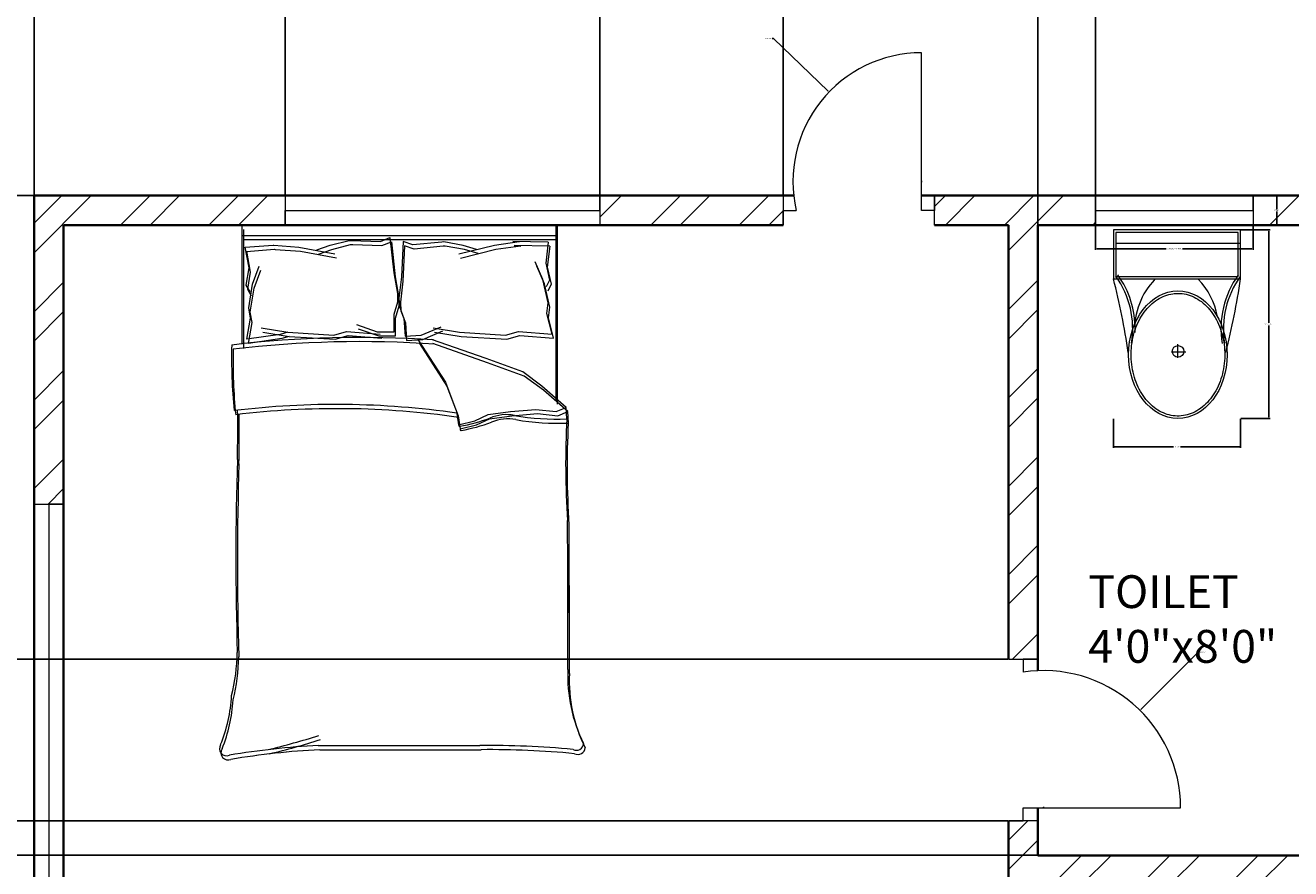
# Model space of a CAD drawing. Units: inches. Extents: x 392 to 1254, y 1207 to 2665.
# Tile 9 of 15: x 540 to 733, y 2127 to 2255. Entities that reach past the tile are written whole.
import ezdxf

# ---------------------------------------------------------------- set-up
doc = ezdxf.new("R2010")
doc.units = ezdxf.units.IN
for name, color, linetype, lineweight in [('A-ANNO-DIMS', 2, 'Continuous', 18), ('A-AREA-IDEN', 7, 'Continuous', 18), ('A-DOOR', 3, 'Continuous', 18), ('A-FLOR-FIXT', 9, 'Continuous', 18), ('A-FURN', 8, 'Continuous', 13), ('A-GLAZ', 4, 'Continuous', 18), ('A-WALL', 7, 'Continuous', 35), ('A-WALL-PATT', 252, 'Continuous', 13)]:
    doc.layers.add(name, color=color, linetype=linetype, lineweight=lineweight)
doc.styles.get("Standard").update_dxf_attribs({"font": 'arial.ttf'})
doc.dimstyles.get("Standard").update_dxf_attribs({"dimtxt": 0.18, "dimasz": 0.18, "dimexe": 0.18, "dimexo": 0.0625, "dimgap": 0.09, "dimtad": 0, "dimtih": 1, "dimtoh": 1, "dimdec": 4, "dimzin": 0, "dimdsep": 46, "dimtxsty": 'Standard', "dimcen": 0.09, "dimadec": 0, "dimazin": 0, "dimtfac": 1, "dimtdec": 4, "dimtofl": 0, "dimtmove": 0, "dimatfit": 3, "dimfxl": 1, "dimtolj": 1, "dimtzin": 0, "dimarcsym": 0})

# ---------------------------------------------------------------- blocks, each defined once
blk = doc.blocks.new('A$C31115884')
for p, q in [((257.5, 466.4), (257.5, 523.2)), ((283.1, 497.7), (223.4, 497.7)), ((0, 200), (0, 0)), ((520, 200), (0, 200)), ((10, 190), (10, 10)), ((510, 190), (10, 190)), ((510, 10), (510, 190)), ((520, 0), (520, 200)), ((510, 54.5), (0, 54.5)), ((10, 10), (510, 10)), ((0, 0), (520, 0))]:
    blk.add_line(p, q)
blk.add_circle((255.6, 496.4), 23.6)
for centre, radius, start, end in [((2777.7, -204.6), 2807, 165.4549, 171.7133), ((3237, 905), 2807, 188.2867, 194.5451), ((-294.5, 403.3), 364.7, 324.2091, 9.3499), ((-294.5, 403.3), 374.7, 324.2091, 9.3499), ((139.5, 406.2), 293.5, 315.8436, 2.6563), ((805.8, 403.3), 364.7, 170.6501, 215.7909), ((805.8, 403.3), 374.7, 179.2036, 215.7909), ((383.6, 406.2), 293.5, 190.2774, 224.1564)]:
    blk.add_arc(centre, radius, start, end)
blk.add_ellipse((256.2, 509.9), major_axis=(0, -260.7), ratio=0.772727)
blk.add_open_spline([(256.2, 259.2), (263.1, 259.2), (270, 259.7), (287.8, 262.3), (298.7, 265.1), (319.9, 273.1), (330.2, 278.4), (350.1, 291.1), (359.7, 298.7), (377.7, 315.9), (386.2, 325.5), (401.7, 346.6), (408.8, 358.1), (421.3, 382.5), (426.8, 395.5), (435.9, 422.4), (439.5, 436.4), (444.8, 465.1), (446.5, 479.7), (447.9, 509.2), (447.6, 524), (445, 553.3), (442.7, 567.8), (436.3, 596), (432.1, 609.7), (421.9, 636), (416, 648.6), (402.5, 672.1), (395, 683), (378.6, 703), (369.8, 712.1), (351.1, 728), (341.3, 734.8), (320.9, 746.2), (310.4, 750.7), (288.9, 757.3), (278, 759.4), (256, 761), (245, 760.6), (223.1, 757.2), (212.3, 754.3), (191.1, 746.1), (180.8, 740.7), (160.9, 727.8), (151.4, 720.1), (133.5, 702.7), (125.1, 693), (109.6, 671.7), (102.6, 660.2), (90.2, 635.7), (84.9, 622.7), (76, 595.6), (72.4, 581.6), (67.2, 552.9), (65.6, 538.2), (64.4, 508.8), (64.8, 494), (67.5, 464.7), (69.9, 450.2), (76.6, 422), (80.8, 408.3), (91.1, 382.2), (97.2, 369.7), (110.8, 346.3), (118.4, 335.4), (134.8, 315.6), (143.7, 306.7), (162.4, 290.9), (172.3, 284.2), (192.8, 273), (203.3, 268.6), (224.8, 262.2), (235.8, 260.2), (249.9, 259.3), (253, 259.2), (256.2, 259.2)], degree=3, knots=[0, 0, 0, 0, 0.110105, 0.110105, 0.285049, 0.285049, 0.459994, 0.459994, 0.634938, 0.634938, 0.809882, 0.809882, 0.984827, 0.984827, 1.159771, 1.159771, 1.334715, 1.334715, 1.50966, 1.50966, 1.684604, 1.684604, 1.859549, 1.859549, 2.034493, 2.034493, 2.209437, 2.209437, 2.384382, 2.384382, 2.559326, 2.559326, 2.73427, 2.73427, 2.909215, 2.909215, 3.084159, 3.084159, 3.259103, 3.259103, 3.434048, 3.434048, 3.608992, 3.608992, 3.783936, 3.783936, 3.958881, 3.958881, 4.133825, 4.133825, 4.30877, 4.30877, 4.483714, 4.483714, 4.658658, 4.658658, 4.833603, 4.833603, 5.008547, 5.008547, 5.183491, 5.183491, 5.358436, 5.358436, 5.53338, 5.53338, 5.708324, 5.708324, 5.883269, 5.883269, 6.058213, 6.058213, 6.233158, 6.233158, 6.283185, 6.283185, 6.283185, 6.283185])
blk = doc.blocks.new('BED-DOUBLE')
for p, q in [((3.47, 63.33), (3.47, 81.44)), ((3.48, 63.33), (3.48, 81.44)), ((51.27, 81.44), (51.27, 54.83)), ((51.27, 81.44), (51.27, 54.83)), ((51.49, 81.44), (51.49, 80.8)), ((3.47, 79.91), (51.27, 79.91)), ((3.48, 79.91), (51.27, 79.91)), ((3.7, 62.69), (3.7, 80.8)), ((3.7, 62.69), (3.7, 80.8)), ((3.7, 79.27), (51.49, 79.27)), ((3.7, 79.27), (51.49, 79.27)), ((16.88, 78.42), (19.77, 79.14)), ((16.88, 78.42), (19.77, 79.14)), ((19.77, 79.14), (20.09, 79.14)), ((19.77, 79.14), (20.09, 79.14)), ((20.09, 79.14), (24.54, 78.99)), ((20.09, 79.14), (24.54, 78.99)), ((24.54, 78.99), (25.98, 79.57)), ((24.54, 78.99), (25.98, 79.57)), ((25.98, 79.57), (26.56, 74.22)), ((25.98, 79.57), (26.56, 74.22)), ((51.49, 80.8), (51.49, 54.19)), ((51.49, 80.8), (51.49, 54.19)), ((3.89, 78.13), (4.47, 74.95)), ((3.89, 78.13), (4.47, 74.95)), ((3.9, 78.1), (8.18, 78.43)), ((3.9, 78.1), (8.18, 78.43)), ((4.12, 77.49), (4.7, 74.31)), ((4.12, 77.49), (4.7, 74.31)), ((4.13, 77.47), (8.41, 77.79)), ((4.13, 77.47), (8.41, 77.79)), ((8.18, 78.43), (8.28, 78.42)), ((8.18, 78.43), (8.28, 78.42)), ((8.28, 78.42), (12.11, 78.13)), ((8.28, 78.42), (12.11, 78.13)), ((8.41, 77.79), (8.51, 77.78)), ((8.41, 77.79), (8.51, 77.78)), ((8.51, 77.78), (12.34, 77.49)), ((8.51, 77.78), (12.34, 77.49)), ((12.11, 78.13), (17.6, 77.11)), ((12.11, 78.13), (17.6, 77.11)), ((12.34, 77.49), (17.83, 76.48)), ((12.34, 77.49), (17.83, 76.48)), ((14.85, 77.69), (16.88, 78.42)), ((14.85, 77.69), (16.88, 78.42)), ((15.08, 77.05), (17.11, 77.78)), ((15.08, 77.05), (17.11, 77.78)), ((17.11, 77.78), (20, 78.5)), ((17.11, 77.78), (20, 78.5)), ((20, 78.5), (20.32, 78.5)), ((20, 78.5), (20.32, 78.5)), ((20.32, 78.5), (24.77, 78.35)), ((20.32, 78.5), (24.77, 78.35)), ((24.77, 78.35), (26.21, 78.93)), ((24.77, 78.35), (26.21, 78.93)), ((26.21, 78.93), (26.79, 73.58)), ((26.21, 78.93), (26.79, 73.58)), ((27.98, 78.95), (27.73, 73.58)), ((27.98, 78.95), (27.73, 73.58)), ((28.21, 78.31), (27.96, 72.94)), ((28.21, 78.31), (27.96, 72.94)), ((29.46, 78.46), (27.98, 78.95)), ((29.46, 78.46), (27.98, 78.95)), ((29.68, 77.82), (28.21, 78.31)), ((29.68, 77.82), (28.21, 78.31)), ((33.88, 78.89), (29.46, 78.46)), ((33.88, 78.89), (29.46, 78.46)), ((34.11, 78.25), (29.68, 77.82)), ((34.11, 78.25), (29.68, 77.82)), ((34.2, 78.91), (33.88, 78.89)), ((34.2, 78.91), (33.88, 78.89)), ((34.43, 78.27), (34.11, 78.25)), ((34.43, 78.27), (34.11, 78.25)), ((37.14, 78.36), (34.2, 78.91)), ((37.14, 78.36), (34.2, 78.91)), ((37.36, 77.73), (34.43, 78.27)), ((37.36, 77.73), (34.43, 78.27)), ((41.91, 78.37), (36.49, 77.02)), ((41.91, 78.37), (36.5, 77.02)), ((42.14, 77.73), (36.72, 76.38)), ((42.14, 77.73), (36.72, 76.38)), ((39.2, 77.77), (37.14, 78.36)), ((39.2, 77.77), (37.14, 78.36)), ((39.43, 77.13), (37.36, 77.73)), ((39.43, 77.13), (37.36, 77.73)), ((45.71, 78.9), (41.91, 78.37)), ((45.71, 78.9), (41.91, 78.37)), ((45.94, 78.26), (42.14, 77.73)), ((45.94, 78.26), (42.14, 77.73)), ((50.11, 78.89), (44.71, 78.98)), ((44.71, 78.98), (45.71, 78.9)), ((50.11, 78.89), (44.71, 78.98)), ((44.71, 78.98), (45.71, 78.9)), ((50.34, 78.25), (44.94, 78.34)), ((44.94, 78.34), (45.94, 78.26)), ((50.34, 78.25), (44.94, 78.34)), ((44.94, 78.34), (45.94, 78.26)), ((50.11, 78.89), (49.73, 75.67)), ((50.11, 78.89), (49.73, 75.67)), ((50.34, 78.25), (49.96, 75.04)), ((50.34, 78.25), (49.96, 75.04)), ((5.05, 72.49), (6.06, 75.23)), ((5.05, 72.49), (6.06, 75.23)), ((49.31, 73.19), (48.13, 75.86)), ((49.31, 73.19), (48.13, 75.86)), ((49.54, 72.55), (48.36, 75.22)), ((49.54, 72.55), (48.36, 75.22)), ((49.73, 75.67), (50.33, 73.1)), ((49.73, 75.67), (50.33, 73.1)), ((4.47, 74.95), (4.04, 72.34)), ((4.47, 74.95), (4.04, 72.34)), ((4.7, 74.31), (4.27, 71.7)), ((4.7, 74.31), (4.27, 71.7)), ((5.28, 71.85), (6.29, 74.6)), ((5.28, 71.85), (6.29, 74.6)), ((26.56, 74.22), (27.14, 71.04)), ((26.56, 74.22), (27.14, 71.04)), ((26.79, 73.58), (27.37, 70.4)), ((26.79, 73.58), (27.37, 70.4)), ((27.73, 73.58), (27.35, 70.36)), ((27.73, 73.58), (27.35, 70.36)), ((49.96, 75.04), (50.56, 72.47)), ((49.96, 75.04), (50.56, 72.47)), ((4.04, 72.34), (4.62, 71.33)), ((4.04, 72.34), (4.62, 71.33)), ((4.27, 71.7), (4.85, 70.69)), ((4.27, 71.7), (4.85, 70.69)), ((4.47, 68.87), (5.05, 72.49)), ((4.47, 68.87), (5.05, 72.49)), ((4.7, 68.23), (5.28, 71.85)), ((4.7, 68.23), (5.28, 71.85)), ((27.96, 72.94), (27.58, 69.73)), ((27.96, 72.94), (27.58, 69.73)), ((50.11, 69.61), (49.31, 73.19)), ((50.11, 69.61), (49.31, 73.19)), ((50.34, 68.97), (49.54, 72.55)), ((50.34, 68.97), (49.54, 72.55)), ((50.33, 73.1), (49.81, 72.06)), ((50.33, 73.1), (49.81, 72.06)), ((50.56, 72.47), (50.04, 71.42)), ((50.56, 72.47), (50.04, 71.42)), ((27.14, 69.74), (26.56, 67.86)), ((27.14, 69.74), (26.56, 67.86)), ((27.14, 71.04), (27.14, 69.74)), ((27.14, 71.04), (27.14, 69.74)), ((27.35, 70.36), (27.44, 69.07)), ((27.35, 70.36), (27.44, 69.07)), ((27.37, 70.4), (27.37, 69.1)), ((27.37, 70.4), (27.37, 69.1)), ((27.58, 69.73), (27.66, 68.43)), ((27.58, 69.73), (27.66, 68.43)), ((49.92, 68.01), (50.11, 69.61)), ((49.92, 68.01), (50.11, 69.61)), ((4.76, 67.28), (4.47, 68.87)), ((4.76, 67.28), (4.47, 68.87)), ((4.99, 66.64), (4.7, 68.23)), ((4.99, 66.64), (4.7, 68.23)), ((26.56, 67.86), (26.56, 65.18)), ((26.56, 67.86), (26.56, 65.18)), ((27.37, 69.1), (26.79, 67.22)), ((27.37, 69.1), (26.79, 67.22)), ((27.44, 69.07), (28.13, 67.23)), ((27.44, 69.07), (28.13, 67.23)), ((27.66, 68.43), (28.36, 66.59)), ((27.66, 68.43), (28.36, 66.59)), ((50.7, 64.87), (49.92, 68.01)), ((50.7, 64.87), (49.92, 68.01)), ((50.15, 67.37), (50.34, 68.97)), ((50.15, 67.37), (50.34, 68.97)), ((4.18, 64.1), (4.76, 67.28)), ((4.18, 64.1), (4.76, 67.28)), ((4.41, 63.46), (4.99, 66.64)), ((4.41, 63.46), (4.99, 66.64)), ((6.38, 65.81), (10.41, 65.15)), ((6.38, 65.81), (10.41, 65.15)), ((24.1, 65.18), (20.96, 66.27)), ((24.1, 65.18), (20.96, 66.27)), ((24.33, 64.54), (21.19, 65.63)), ((24.33, 64.54), (21.19, 65.63)), ((26.79, 67.22), (26.79, 64.54)), ((26.79, 67.22), (26.79, 64.54)), ((28.13, 67.23), (28.3, 64.55)), ((28.13, 67.23), (28.3, 64.55)), ((28.36, 66.59), (28.53, 63.91)), ((28.36, 66.59), (28.53, 63.91)), ((30.75, 64.7), (33.82, 65.99)), ((30.75, 64.7), (33.82, 65.99)), ((32.56, 65.81), (36.6, 65.15)), ((32.56, 65.81), (36.6, 65.15)), ((50.93, 64.23), (50.15, 67.37)), ((50.93, 64.23), (50.15, 67.37)), ((9.28, 64.82), (4.18, 64.1)), ((9.28, 64.82), (4.18, 64.1)), ((9.51, 64.19), (4.41, 63.46)), ((9.51, 64.19), (4.41, 63.46)), ((6.61, 65.17), (10.64, 64.51)), ((6.61, 65.17), (10.64, 64.51)), ((10.41, 65.15), (9.28, 64.82)), ((10.41, 65.15), (9.28, 64.82)), ((10.64, 64.51), (9.51, 64.19)), ((10.64, 64.51), (9.51, 64.19)), ((10.41, 65.15), (17.42, 64.72)), ((10.41, 65.15), (17.42, 64.72)), ((10.64, 64.51), (17.65, 64.08)), ((10.64, 64.51), (17.65, 64.08)), ((17.42, 64.72), (19.38, 65.27)), ((17.42, 64.72), (19.38, 65.27)), ((17.65, 64.08), (19.61, 64.63)), ((17.65, 64.08), (19.61, 64.63)), ((19.38, 65.27), (24.52, 64.87)), ((19.38, 65.27), (24.52, 64.87)), ((19.61, 64.63), (24.74, 64.23)), ((19.61, 64.63), (24.74, 64.23)), ((26.56, 65.18), (24.1, 65.18)), ((26.56, 65.18), (24.1, 65.18)), ((26.79, 64.54), (24.33, 64.54)), ((26.79, 64.54), (24.33, 64.54)), ((28.3, 64.55), (30.75, 64.7)), ((28.3, 64.55), (30.75, 64.7)), ((28.53, 63.91), (30.98, 64.06)), ((28.53, 63.91), (30.98, 64.06)), ((30.26, 64.06), (34.45, 57.57)), ((30.26, 64.06), (34.45, 57.57)), ((30.98, 64.06), (34.05, 65.35)), ((30.98, 64.06), (34.05, 65.35)), ((40.64, 61.13), (32.31, 64.06)), ((40.64, 61.13), (32.31, 64.06)), ((32.79, 65.17), (36.82, 64.51)), ((32.79, 65.17), (36.82, 64.51)), ((36.6, 65.15), (43.61, 64.72)), ((36.6, 65.15), (43.61, 64.72)), ((36.82, 64.51), (43.83, 64.08)), ((36.82, 64.51), (43.83, 64.08)), ((43.61, 64.72), (45.57, 65.27)), ((43.61, 64.72), (45.57, 65.27)), ((43.83, 64.08), (45.79, 64.63)), ((43.83, 64.08), (45.79, 64.63)), ((45.57, 65.27), (50.7, 64.87)), ((45.57, 65.27), (50.7, 64.87)), ((45.79, 64.63), (50.93, 64.23)), ((45.79, 64.63), (50.93, 64.23)), ((30.49, 63.42), (34.68, 56.93)), ((30.49, 63.42), (34.68, 56.93)), ((40.87, 60.49), (32.53, 63.42)), ((40.87, 60.49), (32.53, 63.42)), ((46.22, 59.11), (40.64, 61.13)), ((46.22, 59.11), (40.64, 61.13)), ((46.45, 58.47), (40.87, 60.49)), ((46.45, 58.47), (40.87, 60.49)), ((49.16, 56.95), (46.22, 59.11)), ((49.16, 56.95), (46.22, 59.11)), ((49.39, 56.31), (46.45, 58.47)), ((49.39, 56.31), (46.45, 58.47)), ((34.45, 57.57), (36.15, 53.08)), ((34.45, 57.57), (36.15, 53.08)), ((34.68, 56.93), (36.38, 52.44)), ((34.68, 56.93), (36.38, 52.44)), ((52.87, 53.7), (49.16, 56.95)), ((52.87, 53.7), (49.16, 56.95)), ((53.1, 53.06), (49.39, 56.31)), ((53.1, 53.06), (49.39, 56.31)), ((36.15, 53.08), (36.46, 51.07)), ((36.15, 53.08), (36.46, 51.07)), ((36.38, 52.44), (36.69, 50.43)), ((36.38, 52.44), (36.69, 50.43)), ((38.94, 51.68), (40.95, 52.61)), ((38.94, 51.68), (40.95, 52.61)), ((40.95, 52.61), (44.36, 53.08)), ((40.95, 52.61), (44.36, 53.08)), ((41.18, 51.97), (44.59, 52.44)), ((41.18, 51.97), (44.59, 52.44)), ((44.36, 53.08), (48.23, 53.39)), ((44.36, 53.08), (48.23, 53.39)), ((44.59, 52.44), (48.46, 52.75)), ((44.59, 52.44), (48.46, 52.75)), ((48.23, 53.39), (51.33, 53.08)), ((48.23, 53.39), (51.33, 53.08)), ((48.46, 52.75), (51.56, 52.44)), ((48.46, 52.75), (51.56, 52.44)), ((51.33, 53.08), (52.87, 53.7)), ((51.33, 53.08), (52.87, 53.7)), ((51.56, 52.44), (53.1, 53.06)), ((51.56, 52.44), (53.1, 53.06)), ((52.95, 51.95), (52.87, 53.7, 3.87)), ((52.95, 51.95), (52.87, 53.7, 3.87)), ((53.18, 51.31), (53.1, 53.06, 3.87)), ((53.18, 51.31), (53.1, 53.06, 3.87)), ((36.46, 51.07), (38.94, 51.68)), ((36.46, 51.07), (38.94, 51.68)), ((36.69, 50.43), (39.17, 51.05)), ((36.69, 50.43), (39.17, 51.05)), ((39.17, 51.05), (41.18, 51.97)), ((39.17, 51.05), (41.18, 51.97)), ((15.06, 2.2), (39.68, 2.2)), ((15.06, 2.2), (39.68, 2.2)), ((15.29, 1.56), (39.91, 1.56)), ((15.29, 1.56), (39.91, 1.56))]:
    blk.add_line(p, q)
for centre, radius, start, end in [((21.36, -100.61), 164.97, 86.0865, 96.7821), ((21.36, -100.61), 164.97, 86.0865, 96.7821), ((21.59, -101.25), 164.97, 86.0865, 96.7821), ((21.59, -101.25), 164.97, 86.0865, 96.7821), ((85.16, 61.35), 83.31, 178.7218, 185.604), ((85.16, 61.35), 83.31, 178.7218, 185.604), ((85.39, 60.71), 83.31, 178.7218, 185.604), ((85.39, 60.71), 83.31, 178.7218, 185.604), ((17.76, -74.87), 129.02, 81.7845, 96.9006), ((17.76, -74.87), 129.02, 81.7845, 96.9006), ((17.98, -75.51), 129.02, 81.7845, 96.9006), ((17.98, -75.51), 129.02, 81.7845, 96.9006), ((-167.31, 50.27), 170.11, 358.4762, 1.0082), ((-167.31, 50.27), 170.11, 358.4762, 1.0082), ((-167.08, 49.63), 170.11, 358.4762, 1.0082), ((-167.08, 49.63), 170.11, 358.4762, 1.0082), ((31.15, 79.96), 29.65, 280.6617, 289.8806), ((31.15, 79.96), 29.65, 280.6617, 289.8806), ((43.74, 46.38), 6.22, 78.6608, 113.7384), ((43.74, 46.38), 6.22, 78.6608, 113.7384), ((51.33, 88.1), 36.18, 259.8763, 272.5657), ((51.33, 88.1), 36.18, 259.8763, 272.5657), ((36.64, 51), 0.185, 160.2464, 271.1377), ((36.64, 51), 0.185, 160.2464, 271.1377), ((36.86, 50.36), 0.185, 160.2464, 271.1377), ((36.86, 50.36), 0.185, 160.2464, 271.1377), ((31.38, 79.32), 29.65, 280.6617, 289.8806), ((31.38, 79.32), 29.65, 280.6617, 289.8806), ((43.97, 45.74), 6.22, 78.6608, 113.7384), ((43.97, 45.74), 6.22, 78.6608, 113.7384), ((51.56, 87.46), 36.18, 259.8763, 272.5657), ((51.56, 87.46), 36.18, 259.8763, 272.5657), ((182.27, 45.13), 129.5, 176.9791, 183.8365), ((182.27, 45.13), 129.5, 176.9791, 183.8365), ((182.49, 44.49), 129.5, 176.9791, 183.8365), ((182.49, 44.49), 129.5, 176.9791, 183.8365), ((484.82, 30.83), 482.31, 178.2277, 181.7185), ((484.82, 30.83), 482.31, 178.2277, 181.7185), ((485.05, 30.19), 482.31, 178.2277, 181.7185), ((485.05, 30.19), 482.31, 178.2277, 181.7185), ((-4508.74, 13.62), 4561.86, 0.00217, 0.28689), ((-4508.74, 13.62), 4561.86, 0.00217, 0.28689), ((-4508.51, 12.98), 4561.86, 0.00217, 0.28689), ((-4508.52, 12.98), 4561.86, 0.00217, 0.28689), ((-26.9, 16.93), 29.63, 346.0648, 358.9113), ((-26.9, 16.93), 29.63, 346.0648, 358.9113), ((-26.67, 16.29), 29.63, 346.0648, 358.9113), ((-26.67, 16.29), 29.63, 346.0648, 358.9113), ((76.16, 12.78), 23.07, 177.4714, 206.4681), ((76.16, 12.78), 23.07, 177.4714, 206.4681), ((76.39, 12.14), 23.07, 177.4714, 206.4681), ((76.39, 12.14), 23.07, 177.4714, 206.4681), ((-21.66, 11.17), 23.56, 337.9751, 356.652), ((-21.66, 11.17), 23.56, 337.9751, 356.652), ((-21.43, 10.53), 23.56, 337.9751, 356.652), ((-21.43, 10.53), 23.56, 337.9751, 356.652), ((1.09, 1.72), 1.09, 146.1736, 293.4781), ((1.09, 1.72), 1.09, 146.1736, 293.4781), ((21.43, -119.39), 121.76, 92.9958, 99.4091), ((21.43, -119.39), 121.76, 92.9958, 99.4091), ((-17.22, 105.15), 106.46, 283.3832, 287.7053), ((-17.22, 105.15), 106.46, 283.3832, 287.7053), ((-16.99, 104.52), 106.46, 283.3832, 287.7053), ((-16.99, 104.52), 106.46, 283.3832, 287.7053), ((41.15, -130.83), 133.04, 84.4998, 90.6351), ((41.15, -130.83), 133.04, 84.4998, 90.6351), ((54.41, 2.57), 1.1, 242.6588, 356.02), ((54.41, 2.57), 1.1, 242.6588, 356.02), ((1.32, 1.09), 1.09, 146.1736, 293.4781), ((1.32, 1.09), 1.09, 146.1736, 293.4781), ((21.66, -120.03), 121.76, 92.9958, 99.4091), ((21.65, -120.03), 121.76, 92.9958, 99.4091), ((41.38, -131.47), 133.04, 84.4998, 90.6351), ((41.38, -131.47), 133.04, 84.4998, 90.6351), ((54.64, 1.93), 1.1, 242.6588, 356.02), ((54.64, 1.93), 1.1, 242.6588, 356.02)]:
    blk.add_arc(centre, radius, start, end)
blk = doc.blocks.new('WIN-60-A')
for p, q in [((0, 60), (4.5, 60)), ((4.5, 60), (2.25, 60)), ((2.25, 60), (2.25, 0)), ((2.25, 0), (0, 0)), ((0, 0), (4.5, 0))]:
    blk.add_line(p, q)
blk = doc.blocks.new('WIN-24-A')
for p, q in [((0, 0), (0, 4.5)), ((0, 4.5), (0, 2.25)), ((24, 2.25), (24, 4.5)), ((24, 4.5), (24, 0)), ((0, 2.25), (24, 2.25))]:
    blk.add_line(p, q)
blk = doc.blocks.new('*D13')
at = {"layer": 'A-ANNO-DIMS', "color": 0, "lineweight": -2, "transparency": 16777216}
for p, q in [((725.23, 2224.06), (729.66, 2224.06)), ((729.48, 2223.88), (729.48, 2209.89)), ((729.48, 2195.52), (729.48, 2209.52)), ((725.23, 2195.34), (729.66, 2195.34))]:
    blk.add_line(p, q, dxfattribs=at)
at = {"layer": 'A-ANNO-DIMS', "color": 0, "transparency": 16777216}
for points in [[(729.45, 2223.88), (729.51, 2223.88), (729.48, 2224.06)], [(729.45, 2195.52), (729.51, 2195.52), (729.48, 2195.34)]]:
    blk.add_solid(points, dxfattribs=at)
at = {"layer": 'Defpoints', "color": 0, "transparency": 16777216}
for p in [(725.17, 2224.06), (725.17, 2195.34), (729.48, 2195.34)]:
    blk.add_point(p, dxfattribs=at)
at = {"layer": 'A-ANNO-DIMS', "color": 0, "transparency": 16777216, "insert": (729.48, 2209.7), "char_height": 0.18, "attachment_point": 5}
blk.add_mtext('\\A1;WC 29 TYP.', dxfattribs=at)
blk = doc.blocks.new('*D14')
at = {"layer": 'A-ANNO-DIMS', "color": 0, "lineweight": -2, "transparency": 16777216}
for p, q in [((705.79, 2195.28), (705.79, 2190.85)), ((725.17, 2195.28), (725.17, 2190.85)), ((705.97, 2191.03), (714.96, 2191.03)), ((724.99, 2191.03), (716, 2191.03))]:
    blk.add_line(p, q, dxfattribs=at)
at = {"layer": 'A-ANNO-DIMS', "color": 0, "transparency": 16777216}
for points in [[(705.97, 2191.06), (705.97, 2191), (705.79, 2191.03)], [(724.99, 2191.06), (724.99, 2191), (725.17, 2191.03)]]:
    blk.add_solid(points, dxfattribs=at)
at = {"layer": 'Defpoints', "color": 0, "transparency": 16777216}
for p in [(705.79, 2195.34), (725.17, 2195.34), (705.79, 2191.03)]:
    blk.add_point(p, dxfattribs=at)
at = {"layer": 'A-ANNO-DIMS', "color": 0, "transparency": 16777216, "insert": (715.48, 2191.03), "char_height": 0.18, "attachment_point": 5}
blk.add_mtext('\\A1;19 TYP.', dxfattribs=at)
blk = doc.blocks.new('*D15')
at = {"layer": 'A-ANNO-DIMS', "color": 0, "lineweight": -2, "transparency": 16777216}
for p, q in [((703.08, 2224.73), (703.08, 2221.02)), ((727.08, 2224.73), (727.08, 2221.02)), ((703.26, 2221.2), (713.84, 2221.2)), ((726.9, 2221.2), (716.31, 2221.2))]:
    blk.add_line(p, q, dxfattribs=at)
at = {"layer": 'A-ANNO-DIMS', "color": 0, "transparency": 16777216}
for points in [[(703.26, 2221.23), (703.26, 2221.17), (703.08, 2221.2)], [(726.9, 2221.23), (726.9, 2221.17), (727.08, 2221.2)]]:
    blk.add_solid(points, dxfattribs=at)
at = {"layer": 'Defpoints', "color": 0, "transparency": 16777216}
for p in [(703.08, 2224.8), (727.08, 2224.8), (727.08, 2221.2)]:
    blk.add_point(p, dxfattribs=at)
at = {"layer": 'A-ANNO-DIMS', "color": 0, "transparency": 16777216, "insert": (715.08, 2221.2), "char_height": 0.18, "attachment_point": 5}
blk.add_mtext('\\A1;WINDOW A 24 TYP.', dxfattribs=at)
blk = doc.blocks.new('*D16')
at = {"layer": 'A-ANNO-DIMS', "color": 0, "lineweight": -2, "transparency": 16777216}
for p, q in [((727.14, 2229.3), (730.86, 2229.3)), ((730.68, 2229.12), (730.68, 2227.23)), ((730.68, 2224.98), (730.68, 2226.86)), ((727.14, 2224.8), (730.86, 2224.8))]:
    blk.add_line(p, q, dxfattribs=at)
at = {"layer": 'A-ANNO-DIMS', "color": 0, "transparency": 16777216}
for points in [[(730.65, 2229.12), (730.71, 2229.12), (730.68, 2229.3)], [(730.65, 2224.98), (730.71, 2224.98), (730.68, 2224.8)]]:
    blk.add_solid(points, dxfattribs=at)
at = {"layer": 'Defpoints', "color": 0, "transparency": 16777216}
for p in [(727.08, 2229.3), (730.68, 2229.3), (727.08, 2224.8)]:
    blk.add_point(p, dxfattribs=at)
at = {"layer": 'A-ANNO-DIMS', "color": 0, "transparency": 16777216, "insert": (730.68, 2227.05), "char_height": 0.18, "attachment_point": 5}
blk.add_mtext('\\A1;5 TYP.', dxfattribs=at)
blk = doc.blocks.new('*D26')
at = {"layer": 'A-ANNO-DIMS', "color": 0, "lineweight": -2, "transparency": 16777216}
for p, q in [((541.22, 2229.3), (495, 2229.3)), ((495.18, 2229.12), (495.18, 1819.98)), ((495.18, 1410.48), (495.18, 1819.61)), ((753.23, 1410.3), (495, 1410.3))]:
    blk.add_line(p, q, dxfattribs=at)
at = {"layer": 'A-ANNO-DIMS', "color": 0, "transparency": 16777216}
for points in [[(495.15, 2229.12), (495.21, 2229.12), (495.18, 2229.3)], [(495.15, 1410.48), (495.21, 1410.48), (495.18, 1410.3)]]:
    blk.add_solid(points, dxfattribs=at)
at = {"layer": 'Defpoints', "color": 0, "transparency": 16777216}
for p in [(495.18, 2229.3), (541.28, 2229.3), (753.29, 1410.3)]:
    blk.add_point(p, dxfattribs=at)
at = {"layer": 'A-ANNO-DIMS', "color": 0, "transparency": 16777216, "insert": (495.18, 1819.8), "char_height": 0.18, "attachment_point": 5}
blk.add_mtext('\\A1;819', dxfattribs=at)
blk = doc.blocks.new('*D44')
at = {"layer": 'A-ANNO-DIMS', "color": 0, "lineweight": -2, "transparency": 16777216}
for p, q in [((541.28, 2229.36), (541.28, 2297.33)), ((541.46, 2297.15), (560.01, 2297.15)), ((579.35, 2297.15), (560.8, 2297.15)), ((579.53, 2229.36), (579.53, 2297.33))]:
    blk.add_line(p, q, dxfattribs=at)
at = {"layer": 'A-ANNO-DIMS', "color": 0, "transparency": 16777216}
for points in [[(541.46, 2297.18), (541.46, 2297.12), (541.28, 2297.15)], [(579.35, 2297.18), (579.35, 2297.12), (579.53, 2297.15)]]:
    blk.add_solid(points, dxfattribs=at)
at = {"layer": 'Defpoints', "color": 0, "transparency": 16777216}
for p in [(579.53, 2297.15), (541.28, 2229.3), (579.53, 2229.3)]:
    blk.add_point(p, dxfattribs=at)
at = {"layer": 'A-ANNO-DIMS', "color": 0, "transparency": 16777216, "insert": (560.41, 2297.15), "char_height": 0.18, "attachment_point": 5}
blk.add_mtext('\\A1;38.25', dxfattribs=at)
blk = doc.blocks.new('*D45')
at = {"layer": 'A-ANNO-DIMS', "color": 0, "lineweight": -2, "transparency": 16777216}
for p, q in [((579.53, 2229.36), (579.53, 2297.33)), ((579.71, 2297.15), (603.31, 2297.15)), ((627.35, 2297.15), (603.75, 2297.15)), ((627.53, 2229.36), (627.53, 2297.33))]:
    blk.add_line(p, q, dxfattribs=at)
at = {"layer": 'A-ANNO-DIMS', "color": 0, "transparency": 16777216}
for points in [[(579.71, 2297.18), (579.71, 2297.12), (579.53, 2297.15)], [(627.35, 2297.18), (627.35, 2297.12), (627.53, 2297.15)]]:
    blk.add_solid(points, dxfattribs=at)
at = {"layer": 'Defpoints', "color": 0, "transparency": 16777216}
for p in [(627.53, 2297.15), (579.53, 2229.3), (627.53, 2229.3)]:
    blk.add_point(p, dxfattribs=at)
at = {"layer": 'A-ANNO-DIMS', "color": 0, "transparency": 16777216, "insert": (603.53, 2297.15), "char_height": 0.18, "attachment_point": 5}
blk.add_mtext('\\A1;48', dxfattribs=at)
blk = doc.blocks.new('*D46')
at = {"layer": 'A-ANNO-DIMS', "color": 0, "lineweight": -2, "transparency": 16777216}
for p, q in [((627.53, 2229.36), (627.53, 2297.33)), ((627.71, 2297.15), (641.02, 2297.15)), ((655.26, 2297.15), (641.95, 2297.15)), ((655.44, 2229.36), (655.44, 2297.33))]:
    blk.add_line(p, q, dxfattribs=at)
at = {"layer": 'A-ANNO-DIMS', "color": 0, "transparency": 16777216}
for points in [[(627.71, 2297.18), (627.71, 2297.12), (627.53, 2297.15)], [(655.26, 2297.18), (655.26, 2297.12), (655.44, 2297.15)]]:
    blk.add_solid(points, dxfattribs=at)
at = {"layer": 'Defpoints', "color": 0, "transparency": 16777216}
for p in [(655.44, 2297.15), (627.53, 2229.3), (655.44, 2229.3)]:
    blk.add_point(p, dxfattribs=at)
at = {"layer": 'A-ANNO-DIMS', "color": 0, "transparency": 16777216, "insert": (641.49, 2297.15), "char_height": 0.18, "attachment_point": 5}
blk.add_mtext('\\A1;27.913', dxfattribs=at)
blk = doc.blocks.new('*D76')
at = {"layer": 'A-ANNO-DIMS', "color": 0, "lineweight": -2, "transparency": 16777216}
for p, q in [((694.28, 2224.86), (694.28, 2297.33)), ((694.46, 2297.15), (698.28, 2297.15)), ((702.9, 2297.15), (699.07, 2297.15)), ((703.08, 2224.86), (703.08, 2297.33))]:
    blk.add_line(p, q, dxfattribs=at)
at = {"layer": 'A-ANNO-DIMS', "color": 0, "transparency": 16777216}
for points in [[(694.46, 2297.18), (694.46, 2297.12), (694.28, 2297.15)], [(702.9, 2297.18), (702.9, 2297.12), (703.08, 2297.15)]]:
    blk.add_solid(points, dxfattribs=at)
at = {"layer": 'Defpoints', "color": 0, "transparency": 16777216}
for p in [(703.08, 2297.15), (694.28, 2224.8), (703.08, 2224.8)]:
    blk.add_point(p, dxfattribs=at)
at = {"layer": 'A-ANNO-DIMS', "color": 0, "transparency": 16777216, "insert": (698.68, 2297.15), "char_height": 0.18, "attachment_point": 5}
blk.add_mtext('\\A1;8.795', dxfattribs=at)
blk = doc.blocks.new('*D81')
at = {"layer": 'A-ANNO-DIMS', "color": 0, "lineweight": -2, "transparency": 16777216}
for p, q in [((689.72, 2158.7), (495, 2158.7)), ((495.18, 2158.52), (495.18, 2146.56)), ((495.18, 2134.24), (495.18, 2146.19)), ((689.72, 2134.06), (495, 2134.06))]:
    blk.add_line(p, q, dxfattribs=at)
at = {"layer": 'A-ANNO-DIMS', "color": 0, "transparency": 16777216}
for points in [[(495.15, 2158.52), (495.21, 2158.52), (495.18, 2158.7)], [(495.15, 2134.24), (495.21, 2134.24), (495.18, 2134.06)]]:
    blk.add_solid(points, dxfattribs=at)
at = {"layer": 'Defpoints', "color": 0, "transparency": 16777216}
for p in [(495.18, 2158.7), (689.78, 2158.7), (689.78, 2134.06)]:
    blk.add_point(p, dxfattribs=at)
at = {"layer": 'A-ANNO-DIMS', "color": 0, "transparency": 16777216, "insert": (495.18, 2146.38), "char_height": 0.18, "attachment_point": 5}
blk.add_mtext('\\A1;24.64', dxfattribs=at)
blk = doc.blocks.new('*D82')
at = {"layer": 'A-ANNO-DIMS', "color": 0, "lineweight": -2, "transparency": 16777216}
for p, q in [((689.72, 2134.06), (495, 2134.06)), ((495.18, 2133.88), (495.18, 2131.61)), ((495.18, 2128.98), (495.18, 2131.24)), ((694.22, 2128.8), (495, 2128.8))]:
    blk.add_line(p, q, dxfattribs=at)
at = {"layer": 'A-ANNO-DIMS', "color": 0, "transparency": 16777216}
for points in [[(495.15, 2133.88), (495.21, 2133.88), (495.18, 2134.06)], [(495.15, 2128.98), (495.21, 2128.98), (495.18, 2128.8)]]:
    blk.add_solid(points, dxfattribs=at)
at = {"layer": 'Defpoints', "color": 0, "transparency": 16777216}
for p in [(495.18, 2134.06), (689.78, 2134.06), (694.28, 2128.8)]:
    blk.add_point(p, dxfattribs=at)
at = {"layer": 'A-ANNO-DIMS', "color": 0, "transparency": 16777216, "insert": (495.18, 2131.43), "char_height": 0.18, "attachment_point": 5}
blk.add_mtext('\\A1;5.26', dxfattribs=at)
blk = doc.blocks.new('*D98')
at = {"layer": 'A-ANNO-DIMS', "color": 0, "lineweight": -2, "transparency": 16777216}
for p, q in [((653.79, 2253.22), (653.97, 2253.22)), ((653.97, 2253.22), (662.3, 2245.18)), ((676.44, 2231.46), (676.62, 2231.46)), ((676.53, 2231.37), (676.53, 2231.55))]:
    blk.add_line(p, q, dxfattribs=at)
at = {"layer": 'A-ANNO-DIMS', "color": 0, "transparency": 16777216}
blk.add_solid([(662.32, 2245.2), (662.28, 2245.16), (662.43, 2245.06)], dxfattribs=at)
at = {"layer": 'Defpoints', "color": 0, "transparency": 16777216}
for p in [(662.43, 2245.06), (676.53, 2231.46)]:
    blk.add_point(p, dxfattribs=at)
at = {"layer": 'A-ANNO-DIMS', "color": 0, "transparency": 16777216, "insert": (653.24, 2253.22), "char_height": 0.18, "attachment_point": 5}
blk.add_mtext('\\A1;R19.586', dxfattribs=at)
blk = doc.blocks.new('*D99')
at = {"layer": 'A-ANNO-DIMS', "color": 0, "lineweight": -2, "transparency": 16777216}
for p, q in [((718.7, 2159.75), (709.99, 2150.99)), ((718.88, 2159.75), (718.7, 2159.75)), ((695.06, 2136.06), (695.24, 2136.06)), ((695.15, 2135.97), (695.15, 2136.15))]:
    blk.add_line(p, q, dxfattribs=at)
at = {"layer": 'A-ANNO-DIMS', "color": 0, "transparency": 16777216}
blk.add_solid([(709.97, 2151.02), (710.02, 2150.97), (709.87, 2150.87)], dxfattribs=at)
at = {"layer": 'Defpoints', "color": 0, "transparency": 16777216}
for p in [(709.87, 2150.87), (695.15, 2136.06)]:
    blk.add_point(p, dxfattribs=at)
at = {"layer": 'A-ANNO-DIMS', "color": 0, "transparency": 16777216, "insert": (719.42, 2159.75), "char_height": 0.18, "attachment_point": 5}
blk.add_mtext('\\A1;R20.877', dxfattribs=at)

msp = doc.modelspace()

# ---------------------------------------------------------------- hatches: boundary and pattern name
at = {"layer": 'A-WALL-PATT'}
h = msp.add_hatch(dxfattribs=at)
h.set_pattern_fill('ANSI32', color=256)
h.paths.add_polyline_path([(579.5309, 2227.0453), (579.5309, 2229.2953), (541.2807, 2229.2953), (541.2807, 2182.3091), (545.7807, 2182.3091), (545.7807, 2224.7953), (579.5309, 2224.7953)])
h.paths.add_polyline_path([(655.4442, 2229.2953), (627.5309, 2229.2953), (627.5309, 2224.7953), (655.4442, 2224.7953), (655.4442, 2227.0453)])
h.paths.add_polyline_path([(703.0758, 2229.2953), (678.5257, 2229.2953), (678.5257, 2227.0453), (678.5257, 2224.7953), (689.7807, 2224.7953), (689.7807, 2158.6973), (694.2807, 2158.6973), (694.2807, 2224.7953), (703.0758, 2224.7953)])
h.paths.add_polyline_path([(768.5767, 2229.2953), (727.0758, 2229.2953), (727.0758, 2224.7953), (742.2807, 2224.7953), (742.2807, 2128.7953), (694.2807, 2128.7953), (694.2807, 2134.0554), (689.7807, 2134.0554), (689.7807, 2090.2854), (694.2807, 2090.2854), (694.2807, 2124.2953), (742.2807, 2124.2953), (742.2807, 2052.2953), (795.2124, 2052.2953), (795.2124, 2054.5453), (795.2124, 2056.7953), (746.7807, 2056.7953), (746.7807, 2224.7953), (768.5767, 2224.7953)])
h.paths.add_polyline_path([(867.5089, 2229.2953), (804.5767, 2229.2953), (804.5767, 2224.7953), (830.7807, 2224.7953), (830.7807, 2056.7953), (826.9066, 2056.7953), (826.9066, 2052.2953), (830.7807, 2052.2953), (830.7807, 1886.6777, -0.01766664), (830.8602, 1884.2953), (835.0818, 1884.2953, -0.04411348), (835.2807, 1889.9369), (835.2807, 2052.2953), (839.418, 2052.2953), (839.418, 2056.7953), (835.2807, 2056.7953), (835.2807, 2224.7953), (867.5089, 2224.7953)])
h.paths.add_polyline_path([(939.8604, 2229.2953), (903.5089, 2229.2953), (903.5089, 2227.0453), (903.5089, 2224.7953), (919.2807, 2224.7953), (919.2807, 2056.7953), (870.6499, 2056.7953), (870.6499, 2052.2953), (923.7807, 2052.2953), (923.7807, 2124.2953), (971.7807, 2124.2953), (971.7807, 2089.7112), (974.0307, 2089.7112), (976.2807, 2089.7112), (976.2807, 2133.56), (974.0307, 2133.56), (971.7807, 2133.56), (971.7807, 2128.7953), (923.7807, 2128.7953), (923.7807, 2224.7953), (939.8604, 2224.7953)])
h.paths.add_polyline_path([(1124.7807, 2229.2953), (1009.403, 2229.2953), (1009.403, 2224.7953), (1120.2807, 2224.7953), (1120.2807, 2184.7605), (1124.7807, 2184.7605)])
h.paths.add_polyline_path([(1124.7807, 2124.7605), (1120.2807, 2124.7605), (1120.2807, 2056.7953), (976.2807, 2056.7953), (976.2807, 2061.471), (971.7807, 2061.471), (971.7807, 2047.7483), (974.0307, 2047.7483), (976.2807, 2047.7483), (976.2807, 2052.2953), (1120.2807, 2052.2953), (1120.2807, 1992.457), (1124.7807, 1992.457)])
h.paths.add_polyline_path([(1124.7807, 1932.457), (1122.5307, 1932.457), (1120.2807, 1932.457), (1120.2807, 1884.2953), (976.2807, 1884.2953), (976.2807, 2019.9536), (971.7807, 2019.9536), (971.7807, 1884.2953), (869.0911, 1884.2953), (869.0911, 1879.7953), (971.7807, 1879.7953), (1013.7807, 1879.7953), (1013.7807, 1831.7953), (971.7807, 1831.7953), (971.7807, 1822.3831), (974.0307, 1822.3831), (976.2807, 1822.3831), (976.2807, 1827.2953), (1013.7807, 1827.2953), (1025.6191, 1827.2953), (1025.6191, 1829.5453), (1025.6191, 1831.7953), (1018.2807, 1831.7953), (1018.2807, 1879.7953), (1120.2807, 1879.7953), (1120.2807, 1866.9192), (1124.7807, 1866.9192)])
h.paths.add_polyline_path([(1124.7807, 1842.9192), (1122.5307, 1842.9192), (1120.2807, 1842.9192), (1120.2807, 1831.7953), (1050.2021, 1831.7953), (1050.2021, 1827.2953), (1120.2807, 1827.2953), (1120.2807, 1781.4559), (1124.7807, 1781.4559)])
h.paths.add_polyline_path([(976.2807, 1790.8718), (971.7807, 1790.8718), (971.7807, 1648.3339), (976.2807, 1648.3339), (976.2807, 1654.7953), (1120.2807, 1654.7953), (1120.2807, 1626.3807), (1124.7807, 1626.3807), (1124.7807, 1721.4559), (1120.2807, 1721.4559), (1120.2807, 1659.2953), (976.2807, 1659.2953)])
h.paths.add_polyline_path([(1124.7807, 1566.3807), (1120.2807, 1566.3807), (1120.2807, 1486.7953), (1101.07, 1486.7953), (1101.07, 1482.2953), (1124.7807, 1482.2953)])
h.paths.add_polyline_path([(1041.07, 1484.5453), (1041.07, 1486.7953), (1006.2807, 1486.7953), (1006.2807, 1484.5453), (1006.2807, 1482.2953), (1041.07, 1482.2953)])
h.paths.add_polyline_path([(976.2807, 1617.5497), (974.0307, 1617.5497), (971.7807, 1617.5497), (971.7807, 1599.2953), (965.8041, 1599.2953), (965.8041, 1594.7953), (971.7807, 1594.7953), (971.7807, 1486.7953), (954.1249, 1486.7953), (954.1249, 1482.2953), (981.5717, 1482.2953), (981.5717, 1484.5453), (981.5717, 1486.7953), (976.2807, 1486.7953)])
h.paths.add_polyline_path([(930.1249, 1486.7953), (887.7807, 1486.7953), (887.7807, 1594.7953), (941.9141, 1594.7953), (941.9141, 1597.0453), (941.9141, 1599.2953), (887.7807, 1599.2953), (887.7807, 1659.2953), (863.5916, 1659.2953), (863.5916, 1654.7953), (883.2807, 1654.7953), (883.2807, 1438.7953), (782.7807, 1438.7953), (782.7807, 1486.7953), (782.7807, 1654.7953), (800.1309, 1654.7953), (800.1309, 1657.0453), (800.1309, 1659.2953), (778.2807, 1659.2953), (778.2807, 1599.2953), (721.7333, 1599.2953), (721.7333, 1597.0453), (721.7333, 1594.7953), (778.2807, 1594.7953), (778.2807, 1486.7953), (729.598, 1486.7953), (729.598, 1482.2953), (753.2885, 1482.2953), (753.2885, 1410.2953), (922.9852, 1410.2953), (922.9852, 1482.2953), (930.1249, 1482.2953)])
h.paths.add_polyline_path([(918.4852, 1482.2953), (918.4852, 1414.7953), (757.7885, 1414.7953), (757.7885, 1482.2953), (778.2807, 1482.2953), (778.2807, 1434.2953), (782.7807, 1434.2953), (887.7807, 1434.2953), (887.7807, 1438.7953), (887.7807, 1482.2953)], flags=16)
h.paths.add_polyline_path([(694.2807, 1594.7953), (700.4169, 1594.7953), (700.4169, 1597.0453), (700.4169, 1599.2953), (694.2807, 1599.2953), (694.2807, 1617.7503), (692.0307, 1617.7503), (689.7807, 1617.7503), (689.7807, 1486.7953), (682.7672, 1486.7953), (682.7672, 1482.2953), (705.598, 1482.2953), (705.598, 1484.5453), (705.598, 1486.7953), (694.2807, 1486.7953)])
h.paths.add_polyline_path([(545.7807, 1654.7953), (689.7807, 1654.7953), (689.7807, 1649.7691), (694.2807, 1649.7691), (694.2807, 1789.3981), (692.0307, 1789.3981), (689.7807, 1789.3981), (689.7807, 1659.2953), (545.7807, 1659.2953), (545.7807, 1714.4681), (543.5307, 1714.4681), (541.2807, 1714.4681), (541.2807, 1482.2953), (567.0628, 1482.2953), (567.0628, 1484.5453), (567.0628, 1486.7953), (545.7807, 1486.7953)])
h.paths.add_polyline_path([(545.7807, 1827.2953), (620.2247, 1827.2953), (620.2247, 1829.5453), (620.2247, 1831.7953), (545.7807, 1831.7953), (545.7807, 1846.8518), (541.2807, 1846.8518), (541.2807, 1774.4681), (545.7807, 1774.4681)])
h.paths.add_polyline_path([(797.0944, 1884.2953), (694.2807, 1884.2953), (694.2807, 2019.0288), (692.0307, 2019.0288), (689.7807, 2019.0288), (689.7807, 1884.2953), (545.7807, 1884.2953), (545.7807, 1951.8244), (541.2807, 1951.8244), (541.2807, 1870.8518), (543.5307, 1870.8518), (545.7807, 1870.8518), (545.7807, 1879.7953), (647.7807, 1879.7953), (647.7807, 1831.7953), (642.6413, 1831.7953), (642.6413, 1827.2953), (652.2807, 1827.2953), (689.7807, 1827.2953), (689.7807, 1821.0531), (694.2807, 1821.0531), (694.2807, 1831.7953), (652.2807, 1831.7953), (652.2807, 1879.7953), (797.0944, 1879.7953), (797.0944, 1882.0453)])
h.paths.add_polyline_path([(545.7807, 2122.3091), (541.2807, 2122.3091), (541.2807, 2011.8244), (543.5307, 2011.8244), (545.7807, 2011.8244), (545.7807, 2052.2953), (689.7807, 2052.2953), (689.7807, 2048.2048), (694.2807, 2048.2048), (694.2807, 2061.3129), (692.0307, 2061.3129), (689.7807, 2061.3129), (689.7807, 2056.7953), (545.7807, 2056.7953)])

# ---------------------------------------------------------------- linework, layer by layer
at = {"layer": 'A-DOOR'}
for p, q in [((676.5257, 2227.0453), (676.5257, 2251.0453)), ((655.4442, 2229.2953), (655.4442, 2224.7953)), ((678.5257, 2224.7953), (678.5257, 2229.2953)), ((678.5257, 2229.2953), (678.5257, 2227.0453)), ((655.4442, 2224.7953), (655.4442, 2227.0453)), ((655.4442, 2227.0453), (657.4442, 2227.0453)), ((678.5257, 2227.0453), (676.5257, 2227.0453)), ((689.7807, 2158.6973), (694.2807, 2158.6973)), ((694.2807, 2158.6973), (692.0307, 2158.6973)), ((692.0307, 2158.6973), (692.0307, 2156.6973)), ((692.0307, 2134.0554), (692.0307, 2136.0554)), ((692.0307, 2136.0554), (716.0307, 2136.0554)), ((694.2807, 2134.0554), (689.7807, 2134.0554)), ((689.7807, 2134.0554), (692.0307, 2134.0554))]:
    msp.add_line(p, q, dxfattribs=at)
for centre, radius, start, end in [((676.5257, 2231.4598), 19.5855, 90, 193.026117), ((695.1539, 2136.0554), 20.8768, 0, 98.603727)]:
    msp.add_arc(centre, radius, start, end, dxfattribs=at)
at = {"layer": 'A-GLAZ'}
for p, q in [((579.5309, 2229.2953), (579.5309, 2224.7953)), ((627.5309, 2227.0453), (627.5309, 2229.2953)), ((627.5309, 2229.2953), (627.5309, 2224.7953)), ((579.5309, 2224.7953), (579.5309, 2227.0453)), ((579.5309, 2227.0453), (627.5309, 2227.0453))]:
    msp.add_line(p, q, dxfattribs=at)
at = {"layer": 'A-WALL'}
for p, q in [((541.2807, 2229.2953), (657.0602, 2229.2953)), ((541.2807, 2229.2953), (541.2807, 1482.2953)), ((676.5257, 2229.2953), (985.8869, 2229.2953)), ((545.7807, 2224.7953), (655.4442, 2224.7953)), ((545.7807, 2224.7953), (545.7807, 2056.7953)), ((678.5257, 2224.7953), (689.7807, 2224.7953)), ((689.7807, 2224.7953), (689.7807, 2158.6973)), ((694.2807, 2224.7953), (694.2807, 2156.914)), ((694.2807, 2224.7953), (742.2807, 2224.7953)), ((694.2807, 2136.0554), (694.2807, 2128.7953)), ((689.7807, 2134.0554), (689.7807, 2089.0148)), ((694.2807, 2128.7953), (742.2807, 2128.7953))]:
    msp.add_line(p, q, dxfattribs=at)

# ---------------------------------------------------------------- block references
at = {"layer": 'A-FLOR-FIXT', "xscale": 0.0372717239612423, "yscale": 0.0372717239612423, "zscale": 0.0372717239612423, "rotation": 180}
msp.add_blockref('A$C31115884', (725.17, 2224.0627), dxfattribs=at)
at = {"layer": 'A-FURN'}
msp.add_blockref('BED-DOUBLE', (569.531, 2143.326), dxfattribs=at)
at = {"layer": 'A-GLAZ'}
for name, p in [('WIN-24-A', (703.076, 2224.795)), ('WIN-60-A', (541.281, 2122.309))]:
    msp.add_blockref(name, p, dxfattribs=at)

# ---------------------------------------------------------------- texts
at = {"layer": 'A-AREA-IDEN', "insert": (701.9543, 2171.4633), "char_height": 5, "attachment_point": 1}
msp.add_mtext_dynamic_manual_height_columns('TOILET\\P4\'0"x8\'0"', width=116.599073, gutter_width=12.5, heights=[0], dxfattribs=at)

# ---------------------------------------------------------------- dimensions: what is measured, and where the dimension line sits
at = {"layer": 'A-ANNO-DIMS'}
for base, p1, p2, override, picture, middle in [((579.5309, 2297.1453), (541.2807, 2229.2953), (579.5309, 2229.2953), {"dimdec": 2, "dimlfac": 1, "dimrnd": 0, "dimzin": 0, "dimdsep": 46, "dimlunit": 2}, '*D44', (560.4058, 2297.1453)), ((627.5309, 2297.1453), (579.5309, 2229.2953), (627.5309, 2229.2953), {"dimdec": 0, "dimlfac": 1, "dimrnd": 0, "dimzin": 0, "dimdsep": 46, "dimlunit": 2}, '*D45', (603.5309, 2297.1453)), ((655.4442, 2297.1453), (627.5309, 2229.2953), (655.4442, 2229.2953), {"dimdec": 3, "dimlfac": 1, "dimrnd": 0, "dimzin": 0, "dimdsep": 46, "dimlunit": 2}, '*D46', (641.4875, 2297.1453)), ((703.0758, 2297.1453), (694.2807, 2224.7953), (703.0758, 2224.7953), {"dimdec": 3, "dimlfac": 1, "dimrnd": 0, "dimzin": 0, "dimdsep": 46, "dimlunit": 2}, '*D76', (698.6783, 2297.1453))]:
    dim = msp.add_linear_dim(base=base, p1=p1, p2=p2, dimstyle='Standard', override=override, dxfattribs=at)
    dim.commit()
    dim.dimension.update_dxf_attribs({"geometry": picture, "text_midpoint": middle})
for center, mpoint, picture, middle in [((676.5257, 2231.4598), (662.4296, 2245.0573), '*D98', (653.2422, 2253.2158)), ((695.1539, 2136.0554), (709.8672, 2150.8663), '*D99', (719.4249, 2159.7528))]:
    dim = msp.add_radius_dim(center=center, mpoint=mpoint, dimstyle='Standard', override={"dimdec": 3, "dimlfac": 1, "dimrnd": 0, "dimzin": 0, "dimdsep": 46, "dimlunit": 2}, dxfattribs=at)
    dim.commit()
    dim.dimension.update_dxf_attribs({"geometry": picture, "text_midpoint": middle, "dimtype": 164})
for base, p1, p2, override, picture, middle in [((495.1807, 2229.2953), (753.2885, 1410.2953), (541.2807, 2229.2953), {"dimdec": 0, "dimlfac": 1, "dimrnd": 0, "dimzin": 0, "dimdsep": 46, "dimlunit": 2}, '*D26', (495.1807, 1819.7953)), ((495.1807, 2158.6973), (689.7807, 2134.0554), (689.7807, 2158.6973), {"dimdec": 2, "dimlfac": 1, "dimrnd": 0, "dimzin": 0, "dimdsep": 46, "dimlunit": 2}, '*D81', (495.1807, 2146.3764)), ((495.1807, 2134.0554), (694.2807, 2128.7953), (689.7807, 2134.0554), {"dimdec": 2, "dimlfac": 1, "dimrnd": 0, "dimzin": 0, "dimdsep": 46, "dimlunit": 2}, '*D82', (495.1807, 2131.4254))]:
    dim = msp.add_linear_dim(base=base, p1=p1, p2=p2, angle=90, dimstyle='Standard', override=override, dxfattribs=at)
    dim.commit()
    dim.dimension.update_dxf_attribs({"geometry": picture, "text_midpoint": middle})
for base, p1, p2, angle, text, picture, middle in [((730.6758437734, 2229.2953173571), (727.0758437734, 2224.7953173571), (727.0758437734, 2229.2953173571), 90, '<> TYP.', '*D16', (730.6758437734, 2227.0453173571)), ((729.478, 2195.3422), (725.17, 2224.0627), (725.17, 2195.3422), 270, 'WC <> TYP.', '*D13', (729.478, 2209.7025)), ((705.7887, 2191.0342), (725.17, 2195.3422), (705.7887, 2195.3422), 180, '<> TYP.', '*D14', (715.4793, 2191.0342))]:
    dim = msp.add_linear_dim(base=base, p1=p1, p2=p2, angle=angle, text=text, dimstyle='Standard', override={"dimdec": 0, "dimlfac": 1, "dimrnd": 0, "dimzin": 0, "dimdsep": 46, "dimlunit": 2}, dxfattribs=at)
    dim.commit()
    dim.dimension.update_dxf_attribs({"geometry": picture, "text_midpoint": middle})
dim = msp.add_linear_dim(base=(727.0758, 2221.1953), p1=(703.0758, 2224.7953), p2=(727.0758, 2224.7953), text='WINDOW A <> TYP.', dimstyle='Standard', override={"dimdec": 0, "dimlfac": 1, "dimrnd": 0, "dimzin": 0, "dimdsep": 46, "dimlunit": 2}, dxfattribs=at)
dim.commit()
dim.dimension.update_dxf_attribs({"geometry": '*D15', "text_midpoint": (715.0758, 2221.1953)})

doc.saveas('drawing.dxf')
